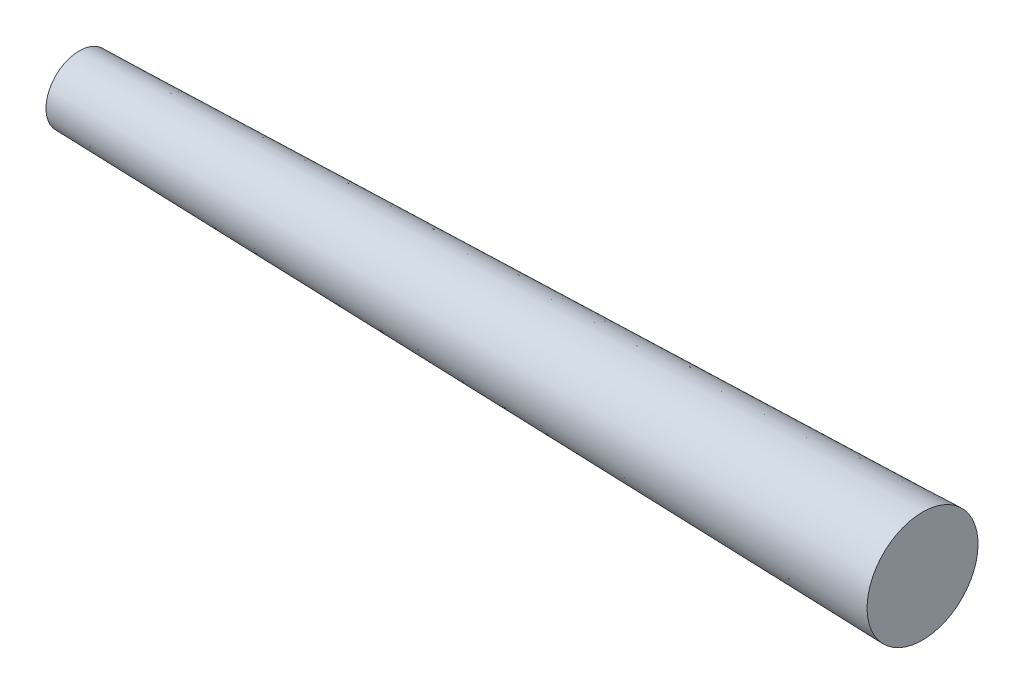
from build123d import *


with BuildPart() as part:
    # Taper Pin Profile → Taper Pin Ø5-Ø3 x 38 (revolve)
    with BuildSketch(Plane.XY):
        Polygon((0, 0), (-38, 0), (-38, 1.5), (0, 2.5), align=None)
    revolve(axis=Axis((0, 0, 0), (-1, 0, 0)))


solid = part.part
